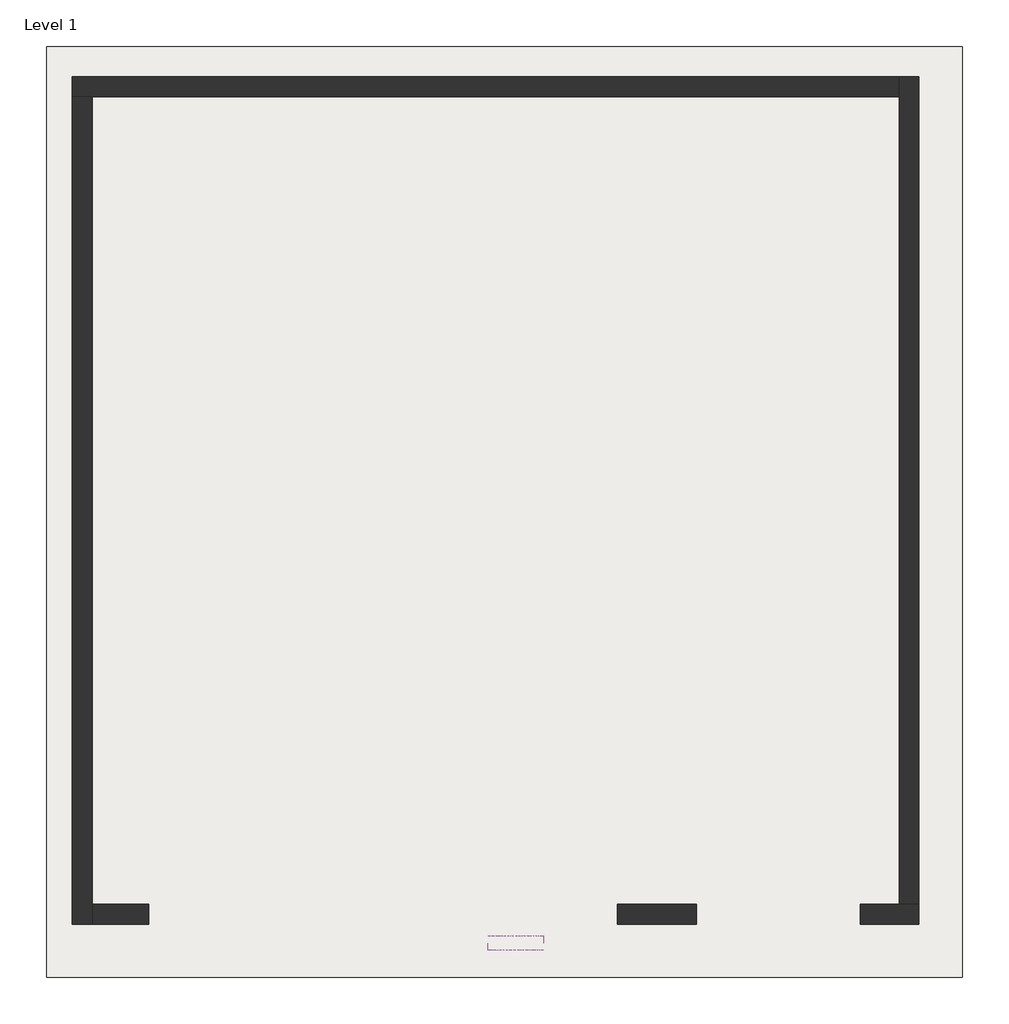
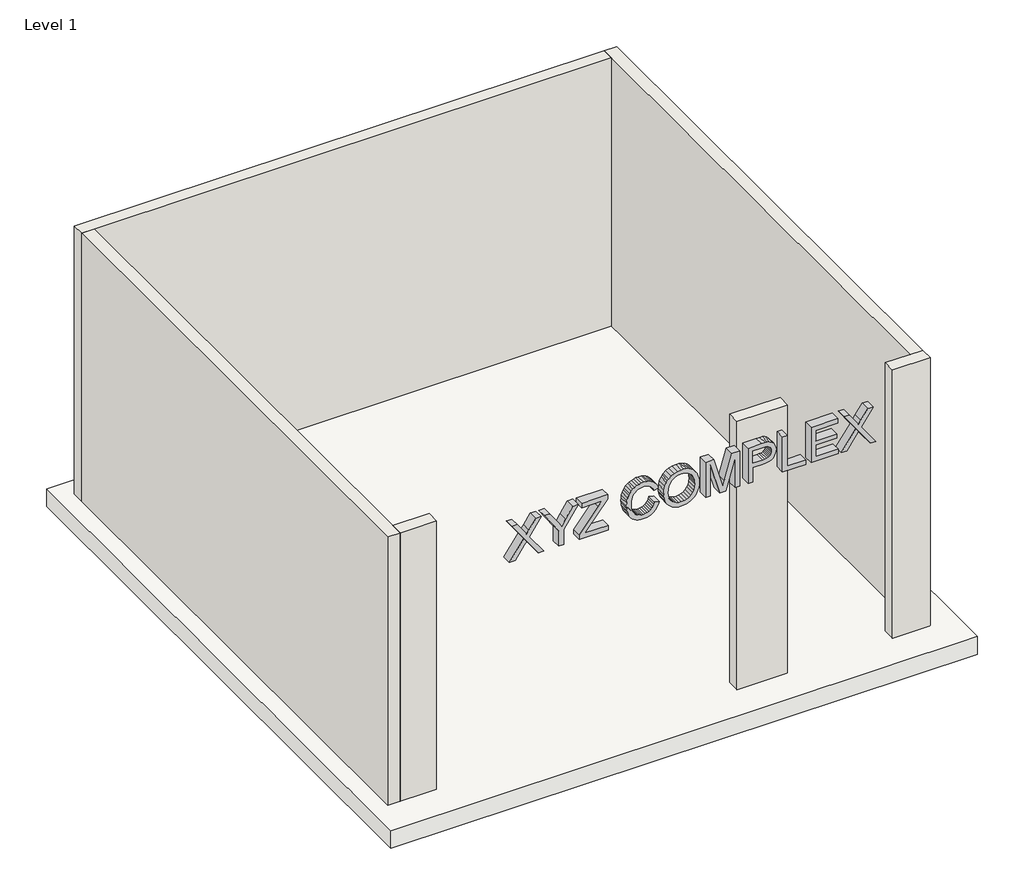
# One storey: 4 walls, 1 proxy, 1 slab.
"""IFC4 building model written with IfcOpenShell, lengths in millimetres."""

from ifc_helpers import new_model, si_unit, frame, origin, place, context, project, spatial, polyline, outline, extrude, faceted_brep, element, save

model = new_model("IFC4")

# Units and contexts
model_context = context("Model", 3, world=origin())
ifc_project = project(units=[si_unit("LENGTHUNIT", "METRE", prefix="MILLI")], contexts=[model_context])

# Site, building, storey
site = spatial("IfcSite", under=ifc_project)
building = spatial("IfcBuilding", under=site)
storey = spatial("IfcBuildingStorey", under=building, Name="Level 1", Elevation=0.0)

# Proxy
placement = place(None, origin())
element("IfcBuildingElementProxy", 1, Name="24\" Arial", ObjectType="24\" Arial", at=placement, inside=storey, context=model_context, shape_type="SweptSolid", body=[
    extrude(outline(polyline([(3672.9507759, -7029.1700033), (3672.9507759, -6937.7300033), (3885.8711605, -6787.2350033), (3935.254622, -6752.212311), (3890.2673143, -6720.1203879), (3672.9507759, -6565.8153879), (3672.9507759, -6475.8407725), (3998.9988528, -6707.2250033), (4273.1723143, -6513.3546186), (4273.1723143, -6604.7946186), (4120.6257759, -6712.7934648), (4059.3726989, -6755.8757725), (4080.4376028, -6766.5364456), (4119.3069297, -6792.6569263), (4273.1723143, -6901.8280802), (4273.1723143, -6991.6561571), (4000.024622, -6797.932311), (3672.9507759, -7029.1700033)])), frame((0.0, 1192.1485991, 0.0), z_axis=(0.0, 1.0, 0.0), x_axis=(0.0, 0.0, 1.0)), (0.0, 0.0, 1.0), 152.4),
    extrude(outline(polyline([(3672.9507759, -6232.0007725), (3672.9507759, -6156.9730802), (3927.1950066, -6156.9730802), (4273.1723143, -5922.5115417), (4273.1723143, -6011.0207725), (4095.1280836, -6124.5880802), (3994.0165451, -6188.9184648), (4088.3873143, -6252.9557725), (4273.1723143, -6378.0996186), (4273.1723143, -6466.462311), (3927.1950066, -6232.0007725), (3672.9507759, -6232.0007725)])), frame((0.0, 1192.1485991, 0.0), z_axis=(0.0, 1.0, 0.0), x_axis=(0.0, 0.0, 1.0)), (0.0, 0.0, 1.0), 152.4),
    extrude(outline(polyline([(3672.9507759, -5903.7546186), (3672.9507759, -5434.8315417), (3747.9784682, -5434.8315417), (3747.9784682, -5811.7284648), (3786.664622, -5780.0761571), (4198.144622, -5444.2100033), (4273.1723143, -5444.2100033), (4273.1723143, -5866.2407725), (4198.144622, -5866.2407725), (4198.144622, -5538.5807725), (4126.7803912, -5596.9030802), (3750.7626989, -5903.7546186), (3672.9507759, -5903.7546186)])), frame((0.0, 1192.1485991, 0.0), z_axis=(0.0, 1.0, 0.0), x_axis=(0.0, 0.0, 1.0)), (0.0, 0.0, 1.0), 152.4),
    extrude(outline(polyline([(3886.3107759, -4693.9330802), (3851.9291893, -4704.1770345), (3822.0536605, -4718.2035129), (3796.6841893, -4736.0125153), (3775.8207759, -4757.6040417), (3759.5366893, -4782.3919384), (3747.9051989, -4809.7900513), (3740.9263047, -4839.7983807), (3738.6000066, -4872.4169263), (3740.3080956, -4899.7692461), (3745.4323624, -4926.1415898), (3753.9728071, -4951.5339576), (3765.9294297, -4975.9463494), (3781.3388648, -4998.2934648), (3800.237747, -5017.4900033), (3822.6260763, -5033.5359648), (3848.5038528, -5046.4313494), (3877.2986605, -5056.3364336), (3908.4380836, -5063.4114936), (3977.7507759, -5069.0715417), (4034.3512566, -5064.2907244), (4089.2665451, -5049.9482725), (4114.9290932, -5038.6327557), (4137.8440451, -5023.8094744), (4158.0114009, -5005.4784287), (4175.4311605, -4983.6396186), (4189.4713768, -4958.6090177), (4199.5001028, -4930.7025994), (4205.5173384, -4899.9203638), (4207.5230836, -4866.262311), (4205.7142494, -4837.0095706), (4200.287747, -4810.3578879), (4191.2435763, -4786.3072629), (4178.5817374, -4764.8576956), (4161.96336, -4745.8992821), (4141.0495739, -4729.3221186), (4115.8403792, -4715.1262052), (4086.3357759, -4703.3115417), (4104.2134682, -4628.2838494), (4144.2551028, -4642.5392941), (4179.5342374, -4661.419859), (4210.050872, -4684.9255441), (4235.8050066, -4713.0563494), (4256.2562807, -4745.281073), (4270.8643336, -4781.0685129), (4279.6291653, -4820.4186691), (4282.5507759, -4863.3315417), (4280.2931677, -4901.8528398), (4273.5203432, -4938.7255802), (4262.2323023, -4973.9497629), (4246.4290451, -5007.5253879), (4226.2754273, -5038.4037893), (4201.9363047, -5065.5363013), (4173.4116773, -5088.9229239), (4140.7015451, -5108.5636571), (4104.4057999, -5124.110472), (4065.1243336, -5135.2153398), (4022.8571461, -5141.8782605), (3977.6042374, -5144.099234), (3935.4286364, -5142.1347028), (3894.6268336, -5136.241109), (3855.1988287, -5126.4184528), (3817.144622, -5112.666734), (3781.9845499, -5095.1553879), (3751.2389489, -5074.0538494), (3724.9078191, -5049.3621186), (3702.9911605, -5021.0801956), (3685.7454153, -4988.7638855), (3673.4270259, -4951.9689936), (3666.0359922, -4910.6955201), (3663.5723143, -4864.9434648), (3666.8282158, -4820.2858686), (3676.5959201, -4779.2184648), (3692.8754273, -4741.7412533), (3715.6667374, -4707.854234), (3744.6584561, -4678.2259888), (3779.5391893, -4653.5250994), (3820.3089369, -4633.7515658), (3866.9676989, -4618.9053879), (3886.3107759, -4693.9330802)])), frame((0.0, 1192.1485991, 0.0), z_axis=(0.0, 1.0, 0.0), x_axis=(0.0, 0.0, 1.0)), (0.0, 0.0, 1.0), 152.4),
    extrude(outline(polyline([(3965.1484682, -4543.8776956), (3926.247086, -4541.7345706), (3888.3806316, -4535.3051956), (3851.5491052, -4524.5895706), (3815.7525066, -4509.5876956), (3782.3325787, -4490.4277917), (3752.6310643, -4467.2380802), (3726.6479634, -4440.018561), (3704.3832759, -4408.769234), (3686.5284802, -4374.3876475), (3673.7750547, -4337.7713494), (3666.1229994, -4298.9203398), (3663.5723143, -4257.8346186), (3665.8802951, -4219.5193903), (3672.8042374, -4182.5321667), (3684.3441412, -4146.872948), (3700.5000066, -4112.541734), (3721.1436124, -4080.7886811), (3746.1467374, -4052.8639456), (3775.5093816, -4028.7675273), (3809.2315451, -4008.4994263), (3846.3332518, -3992.4397268), (3885.8345259, -3980.9685129), (3927.7353672, -3974.0857845), (3972.0357759, -3971.7915417), (4015.7591893, -3973.9713013), (4057.1013528, -3980.5105802), (4096.0622662, -3991.4093783), (4132.6419297, -4006.6676956), (4166.0801749, -4026.0840417), (4195.6168336, -4049.4569263), (4221.2519057, -4076.7863494), (4242.9853912, -4108.072311), (4260.295247, -4142.3531523), (4272.6594297, -4178.6672148), (4280.0779393, -4217.0144985), (4282.5507759, -4257.3950033), (4277.2845499, -4317.7230561), (4261.485872, -4372.2445225), (4235.1547422, -4420.9594023), (4198.2911605, -4463.8676956), (4176.216515, -4482.6200393), (4152.1223864, -4498.8720706), (4097.8756797, -4523.8751956), (4035.5510403, -4538.8770706), (3965.1484682, -4543.8776956)]), holes=[polyline([(3964.4157759, -4468.8500033), (4025.2338167, -4464.9392581), (4076.6825547, -4453.2070225), (4118.7619898, -4433.6532965), (4151.472122, -4406.2780802), (4175.9944177, -4373.4809408), (4193.5103432, -4337.6614456), (4204.0198985, -4298.8195946), (4207.5230836, -4256.9553879), (4205.7050908, -4227.1577076), (4200.2511124, -4198.8712052), (4191.1611485, -4172.0958807), (4178.4351989, -4146.831734), (4162.4029754, -4123.7931403), (4143.3941893, -4103.6944744), (4121.4088408, -4086.5357364), (4096.4469297, -4072.3169263), (4068.870223, -4061.161686), (4039.0404874, -4053.1936571), (4006.957723, -4048.4128398), (3972.6219297, -4046.819234), (3919.7673384, -4050.5422268), (3873.3054874, -4061.7112052), (3833.2363768, -4080.3261691), (3799.5600066, -4106.3871186), (3772.8900066, -4138.2180201), (3753.8400066, -4174.1428398), (3742.4100066, -4214.1615778), (3738.6000066, -4258.274234), (3742.373372, -4301.6450393), (3753.6934682, -4341.196686), (3772.5602951, -4376.9291739), (3798.9738528, -4408.8425033), (3831.9541653, -4435.0957845), (3870.5212566, -4453.8481283), (3914.6751268, -4465.0995345), (3964.4157759, -4468.8500033)])]), frame((0.0, 1192.1485991, 0.0), z_axis=(0.0, 1.0, 0.0), x_axis=(0.0, 0.0, 1.0)), (0.0, 0.0, 1.0), 152.4),
    extrude(outline(polyline([(3672.9507759, -3868.6284648), (3672.9507759, -3793.6007725), (4198.144622, -3793.6007725), (3672.9507759, -3642.6661571), (3672.9507759, -3541.1150033), (4198.144622, -3390.3269263), (3672.9507759, -3390.3269263), (3672.9507759, -3315.299234), (4273.1723143, -3315.299234), (4273.1723143, -3444.3996186), (3857.4426989, -3565.147311), (3761.7530836, -3591.9638494), (3850.1157759, -3616.8753879), (4273.1723143, -3739.9676956), (4273.1723143, -3868.6284648), (3672.9507759, -3868.6284648)])), frame((0.0, 1192.1485991, 0.0), z_axis=(0.0, 1.0, 0.0), x_axis=(0.0, 0.0, 1.0)), (0.0, 0.0, 1.0), 152.4),
    extrude(outline(polyline([(3672.9507759, -3184.0007725), (3672.9507759, -3108.9730802), (3916.7907759, -3108.9730802), (3916.7907759, -2956.4265417), (3920.1062086, -2898.2736691), (3930.0525066, -2849.8381283), (3946.6296701, -2811.1199191), (3969.8376989, -2782.1190417), (3997.8357037, -2760.9946066), (4028.7827951, -2745.9057244), (4062.678973, -2736.8523951), (4099.5242374, -2733.8346186), (4142.2585162, -2738.3040417), (4181.3659682, -2751.712311), (4214.5202951, -2772.4658206), (4239.3951989, -2798.9709648), (4256.7783239, -2831.8871667), (4267.4573143, -2871.8738494), (4271.7435643, -2909.7540417), (4273.1723143, -2961.5553879), (4273.1723143, -3184.0007725), (3672.9507759, -3184.0007725)]), holes=[polyline([(3991.8184682, -3108.9730802), (4198.144622, -3108.9730802), (4198.144622, -2953.7888494), (4196.8624105, -2907.7025033), (4193.0157759, -2878.7611571), (4180.4134682, -2850.4242821), (4159.0188528, -2828.1321186), (4130.5903912, -2813.6797629), (4096.8865451, -2808.862311), (4073.3030114, -2810.9046908), (4052.5220259, -2817.0318302), (4034.5435884, -2827.2437292), (4019.3676989, -2841.5403879), (4007.3149105, -2860.7002917), (3998.7057759, -2885.5019263), (3993.5402951, -2915.9452917), (3991.8184682, -2952.0303879), (3991.8184682, -3108.9730802)])]), frame((0.0, 1192.1485991, 0.0), z_axis=(0.0, 1.0, 0.0), x_axis=(0.0, 0.0, 1.0)), (0.0, 0.0, 1.0), 152.4),
    extrude(outline(polyline([(3672.9507759, -2630.6715417), (3672.9507759, -2255.5330802), (3747.9784682, -2255.5330802), (3747.9784682, -2555.6438494), (4273.1723143, -2555.6438494), (4273.1723143, -2630.6715417), (3672.9507759, -2630.6715417)])), frame((0.0, 1192.1485991, 0.0), z_axis=(0.0, 1.0, 0.0), x_axis=(0.0, 0.0, 1.0)), (0.0, 0.0, 1.0), 152.4),
    extrude(outline(polyline([(3672.9507759, -2171.1269263), (3672.9507759, -1730.339234), (3747.9784682, -1730.339234), (3747.9784682, -2096.099234), (3944.9261605, -2096.099234), (3944.9261605, -1758.4746186), (4019.9538528, -1758.4746186), (4019.9538528, -2096.099234), (4198.144622, -2096.099234), (4198.144622, -1739.7176956), (4273.1723143, -1739.7176956), (4273.1723143, -2171.1269263), (3672.9507759, -2171.1269263)])), frame((0.0, 1192.1485991, 0.0), z_axis=(0.0, 1.0, 0.0), x_axis=(0.0, 0.0, 1.0)), (0.0, 0.0, 1.0), 152.4),
    extrude(outline(polyline([(3672.9507759, -1683.4469263), (3672.9507759, -1592.0069263), (3885.8711605, -1441.5119263), (3935.254622, -1406.489234), (3890.2673143, -1374.397311), (3672.9507759, -1220.092311), (3672.9507759, -1130.1176956), (3998.9988528, -1361.5019263), (4273.1723143, -1167.6315417), (4273.1723143, -1259.0715417), (4120.6257759, -1367.0703879), (4059.3726989, -1410.1526956), (4080.4376028, -1420.8133686), (4119.3069297, -1446.9338494), (4273.1723143, -1556.1050033), (4273.1723143, -1645.9330802), (4000.024622, -1452.209234), (3672.9507759, -1683.4469263)])), frame((0.0, 1192.1485991, 0.0), z_axis=(0.0, 1.0, 0.0), x_axis=(0.0, 0.0, 1.0)), (0.0, 0.0, 1.0), 152.4),
])

# Slab
element("IfcSlab", 2, ObjectType="Generic - 12\"", at=placement, inside=storey, context=model_context, shape_type="SweptSolid", body=[
    extrude(outline(polyline([(349.1590536, 10515.6933455), (349.1590536, 914.4933455), (-9099.6409464, 914.4933455), (-9099.6409464, 10515.6933455), (349.1590536, 10515.6933455)])), frame((0.0, 0.0, -304.8), z_axis=(0.0, 0.0, 1.0), x_axis=(1.0, 0.0, 0.0)), (0.0, 0.0, 1.0), 304.8),
])

# Walls
element("IfcWall", 3, ObjectType="Generic - 8\"", at=placement, inside=storey, context=model_context, shape_type="Brep", body=[
    faceted_brep([(-8833.9561565, 9999.5985991, 0.0), (-8630.7561565, 9999.5985991, 0.0), (-299.5561565, 9999.5985991, 0.0), (-299.5561565, 9999.5985991, 4572.0), (-8630.7561565, 9999.5985991, 4572.0), (-8833.9561565, 9999.5985991, 4572.0), (-8833.9561565, 10202.7985991, 0.0), (-8833.9561565, 10202.7985991, 4572.0), (-299.5561565, 10202.7985991, 4572.0), (-299.5561565, 10202.7985991, 0.0)], [[[0, 1, 2, 3, 4, 5]], [[6, 7, 8, 9]], [[2, 1, 0, 6, 9]], [[0, 5, 7, 6]], [[3, 2, 9, 8]], [[5, 4, 3, 8, 7]]]),
])
element("IfcWall", 4, ObjectType="Generic - 8\"", at=placement, inside=storey, context=model_context, shape_type="Brep", body=[
    faceted_brep([(-8630.7561565, 1465.1985991, 0.0), (-8630.7561565, 1668.3985991, 0.0), (-8630.7561565, 9999.5985991, 0.0), (-8630.7561565, 9999.5985991, 4572.0), (-8630.7561565, 1668.3985991, 4572.0), (-8630.7561565, 1471.5485991, 4572.0), (-8630.7561565, 1465.1985991, 4572.0), (-8833.9561565, 1465.1985991, 0.0), (-8833.9561565, 1465.1985991, 4572.0), (-8833.9561565, 9999.5985991, 4572.0), (-8833.9561565, 9999.5985991, 0.0)], [[[0, 1, 2, 3, 4, 5, 6]], [[7, 8, 9, 10]], [[2, 1, 0, 7, 10]], [[0, 6, 8, 7]], [[3, 2, 10, 9]], [[6, 5, 4, 3, 9, 8]]]),
])
element("IfcWall", 5, ObjectType="Generic - 8\"", at=placement, inside=storey, context=model_context, shape_type="Brep", body=[
    faceted_brep([(-3206.3349032, 1668.3985991, 0.0), (-3206.3349032, 1668.3985991, 4572.0), (-2395.3993702, 1668.3985991, 4572.0), (-2395.3993702, 1668.3985991, 0.0), (-3206.3349032, 1465.1985991, 0.0), (-2395.3993702, 1465.1985991, 0.0), (-2395.3993702, 1465.1985991, 4572.0), (-3206.3349032, 1465.1985991, 4572.0)], [[[0, 1, 2, 3]], [[4, 5, 6, 7]], [[1, 0, 4, 7]], [[3, 2, 6, 5]], [[0, 3, 5, 4]], [[2, 1, 7, 6]]]),
    faceted_brep([(-8630.7561565, 1668.3985991, 4572.0), (-8046.0599727, 1668.3985991, 4572.0), (-8046.0599727, 1668.3985991, 0.0), (-8630.7561565, 1668.3985991, 0.0), (-8630.7561565, 1465.1985991, 4572.0), (-8630.7561565, 1465.1985991, 0.0), (-8046.0599727, 1465.1985991, 0.0), (-8046.0599727, 1465.1985991, 4572.0)], [[[0, 1, 2, 3]], [[4, 5, 6, 7]], [[0, 3, 5, 4]], [[2, 1, 7, 6]], [[3, 2, 6, 5]], [[1, 0, 4, 7]]]),
    faceted_brep([(-96.3561565, 1668.3985991, 4572.0), (-96.3561565, 1668.3985991, 0.0), (-299.5561565, 1668.3985991, 0.0), (-703.8003363, 1668.3985991, 0.0), (-703.8003363, 1668.3985991, 4572.0), (-299.5561565, 1668.3985991, 4572.0), (-96.3561565, 1465.1985991, 0.0), (-96.3561565, 1465.1985991, 4572.0), (-703.8003363, 1465.1985991, 4572.0), (-703.8003363, 1465.1985991, 0.0)], [[[0, 1, 2, 3, 4, 5]], [[6, 7, 8, 9]], [[3, 2, 1, 6, 9]], [[4, 3, 9, 8]], [[0, 5, 4, 8, 7]], [[0, 7, 6, 1]]]),
])
element("IfcWall", 6, ObjectType="Generic - 8\"", at=placement, inside=storey, context=model_context, shape_type="Brep", body=[
    faceted_brep([(-299.5561565, 10202.7985991, 0.0), (-299.5561565, 9999.5985991, 0.0), (-299.5561565, 1668.3985991, 0.0), (-299.5561565, 1668.3985991, 4572.0), (-299.5561565, 9999.5985991, 4572.0), (-299.5561565, 10202.7985991, 4572.0), (-96.3561565, 10202.7985991, 0.0), (-96.3561565, 10202.7985991, 4572.0), (-96.3561565, 1668.3985991, 4572.0), (-96.3561565, 1668.3985991, 0.0)], [[[0, 1, 2, 3, 4, 5]], [[6, 7, 8, 9]], [[2, 1, 0, 6, 9]], [[0, 5, 7, 6]], [[5, 4, 3, 8, 7]], [[2, 9, 8, 3]]]),
])

save(model, "model.ifc")

# Revit data of these elements
# Type "Generic - 12\""
#   Assembly Code = "B1010"
#   Function = 0
#   Layers, outside or top first: 1' - 0" no material (function 1)
# Type "Generic - 8\""
#   Assembly Code = "B2010"
#   Layers, outside or top first: 0' - 8" no material (function 1)
# Element 1 (IfcBuildingElementProxy, "24\" Arial")
#   Phase Created = New Construction
# Element 2 (IfcSlab, "Generic - 12\"")
#   Height Offset From Level = 0' - 0"
#   Phase Created = New Construction
#   Materials on its faces: "Default Floor"
# Elements 3, 4, 5, 6 (IfcWall, "Generic - 8\"")
#   Top Offset = 0' - 0"
#   Base Offset = 0' - 0"
#   Unconnected Height = 12' - 0"
#   wall height = 12' - 0"
#   Phase Created = New Construction
#   Base Constraint = Level 1
#   Materials on its faces: "Default Wall"
# Materials
#   "Default Floor": colour RGB 128 128 128, transparency 0
#   "Default Wall": colour RGB 128 128 128, transparency 0
